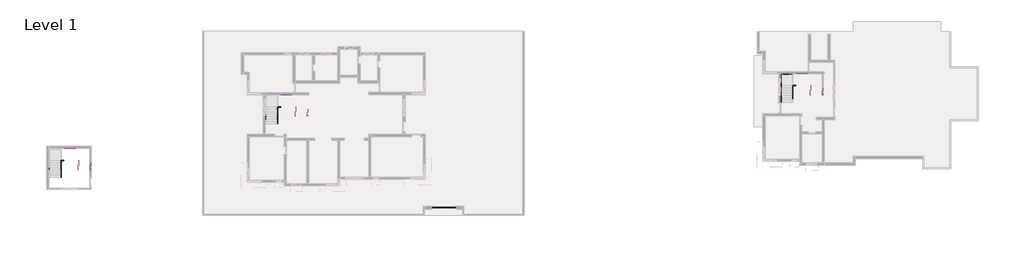
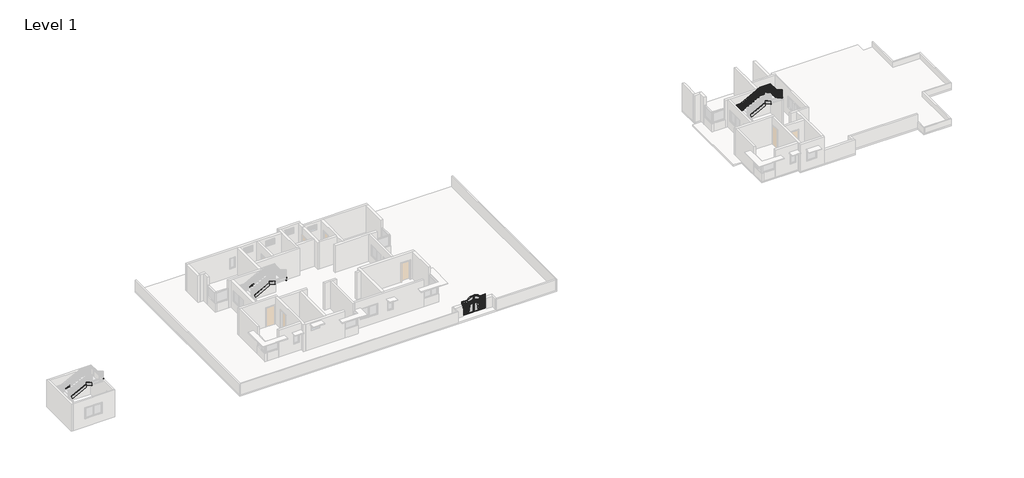
# One storey, part 9 of 9: 18 members, 1 proxy, 1 railing.
"""IFC4 building model written with IfcOpenShell, lengths in millimetres."""

from ifc_helpers import new_model, si_unit, frame, origin, place, context, project, spatial, polyline, outline, extrude, faceted_brep, transform, mapped, element, save
from components import generic_models_6bc30956

model = new_model("IFC4")

# Units and contexts
model_context = context("Model", 3, world=origin())
ifc_project = project(units=[si_unit("LENGTHUNIT", "METRE", prefix="MILLI")], contexts=[model_context])

# Site, building, storey
site = spatial("IfcSite", under=ifc_project)
building = spatial("IfcBuilding", under=site)
storey = spatial("IfcBuildingStorey", under=building, Name="Level 1", Elevation=0.0)

# Proxy
placement = place(None, origin())
generic_models_shape = generic_models_6bc30956(model_context)
element("IfcBuildingElementProxy", 1, Name="Generic Models", at=placement, inside=storey, context=model_context, shape_type="MappedRepresentation", body=[
    mapped(generic_models_shape, transform((-22180.3146233, 3588.8624892, 0.0), x_axis=(1.0, 0.0, 0.0), y_axis=(0.0, 1.0, 0.0), z_axis=(0.0, 0.0, 1.0))),
])

# Members
element("IfcMember", 2, ObjectType="Stringer - 2\" Width", at=placement, inside=storey, context=model_context, shape_type="SweptSolid", body=[
    extrude(outline(polyline([(14647.8480703, 0.0), (14647.8480703, 208.974685), (15536.2673716, 716.6428571), (16150.6114121, 716.6428571), (14896.4864121, 0.0), (14647.8480703, 0.0)])), frame((13242.1100959, 0.0, 0.0), z_axis=(1.0, 0.0, 0.0), x_axis=(0.0, 1.0, 0.0)), (0.0, 0.0, 1.0), 50.8),
])
element("IfcMember", 3, ObjectType="Stringer - 2\" Width", at=placement, inside=storey, context=model_context, shape_type="SweptSolid", body=[
    extrude(outline(polyline([(1570.6066619, 15541.7922297), (1834.574685, 16036.732273), (1834.574685, 15389.032273), (1570.6066619, 14894.0922297), (1570.6066619, 15541.7922297)])), frame((0.0, 17645.0480703, 0.0), z_axis=(0.0, 1.0, 0.0), x_axis=(0.0, 0.0, 1.0)), (0.0, 0.0, 1.0), 50.8),
])
element("IfcMember", 4, ObjectType="Stringer - 2\" Width", at=placement, inside=storey, context=model_context, shape_type="SweptSolid", body=[
    extrude(outline(polyline([(15537.7647285, 2687.6828571), (15409.8480703, 2760.7780904), (15409.8480703, 3111.8318278), (16152.108769, 2687.6828571), (15537.7647285, 2687.6828571)])), frame((17636.3100959, 0.0, 0.0), z_axis=(1.0, 0.0, 0.0), x_axis=(0.0, 1.0, 0.0)), (0.0, 0.0, 1.0), 50.8),
])
element("IfcMember", 5, ObjectType="Stringer - 2\" Width", at=placement, inside=storey, context=model_context, shape_type="SweptSolid", body=[
    extrude(outline(polyline([(14647.8480703, 0.0), (14647.8480703, 208.974685), (16375.0480703, 1195.9461135), (16375.0480703, 844.8923761), (14896.4864121, 0.0), (14647.8480703, 0.0)])), frame((14512.1100959, 0.0, 0.0), z_axis=(1.0, 0.0, 0.0), x_axis=(0.0, 1.0, 0.0)), (0.0, 0.0, 1.0), 50.8),
])
element("IfcMember", 6, ObjectType="Stringer - 2\" Width", at=placement, inside=storey, context=model_context, shape_type="SweptSolid", body=[
    extrude(outline(polyline([(1366.8828571, 14512.1100959), (1021.4428571, 14512.1100959), (2010.3495238, 16366.3100959), (2355.7895238, 16366.3100959), (1366.8828571, 14512.1100959)])), frame((0.0, 16375.0480703, 0.0), z_axis=(0.0, 1.0, 0.0), x_axis=(0.0, 0.0, 1.0)), (0.0, 0.0, 1.0), 50.8),
])
element("IfcMember", 7, ObjectType="Stringer - 2\" Width", at=placement, inside=storey, context=model_context, shape_type="SweptSolid", body=[
    extrude(outline(polyline([(16425.8480703, 2531.2603992), (16425.8480703, 2180.2066619), (15409.8480703, 2760.7780904), (15409.8480703, 3111.8318278), (16425.8480703, 2531.2603992)])), frame((16366.3100959, 0.0, 0.0), z_axis=(1.0, 0.0, 0.0), x_axis=(0.0, 1.0, 0.0)), (0.0, 0.0, 1.0), 50.8),
])
element("IfcMember", 8, ObjectType="Stringer - 2\" Width", at=placement, inside=storey, context=model_context, shape_type="SweptSolid", body=[
    extrude(outline(polyline([(12415.3624892, 0.0), (12415.3624892, 208.974685), (13303.7817906, 716.6428571), (13918.125831, 716.6428571), (12664.000831, 0.0), (12415.3624892, 0.0)])), frame((-41001.7146233, 0.0, 0.0), z_axis=(1.0, 0.0, 0.0), x_axis=(0.0, 1.0, 0.0)), (0.0, 0.0, 1.0), 50.8),
])
element("IfcMember", 9, ObjectType="Stringer - 2\" Width", at=placement, inside=storey, context=model_context, shape_type="SweptSolid", body=[
    extrude(outline(polyline([(1570.6066619, -38702.0324895), (1834.574685, -38207.0924462), (1834.574685, -38854.7924462), (1570.6066619, -39349.7324895), (1570.6066619, -38702.0324895)])), frame((0.0, 15412.5624892, 0.0), z_axis=(0.0, 1.0, 0.0), x_axis=(0.0, 0.0, 1.0)), (0.0, 0.0, 1.0), 50.8),
])
element("IfcMember", 10, ObjectType="Stringer - 2\" Width", at=placement, inside=storey, context=model_context, shape_type="SweptSolid", body=[
    extrude(outline(polyline([(13305.2791475, 2687.6828571), (13177.3624892, 2760.7780904), (13177.3624892, 3111.8318278), (13919.6231879, 2687.6828571), (13305.2791475, 2687.6828571)])), frame((-36607.5146233, 0.0, 0.0), z_axis=(1.0, 0.0, 0.0), x_axis=(0.0, 1.0, 0.0)), (0.0, 0.0, 1.0), 50.8),
])
element("IfcMember", 11, ObjectType="Stringer - 2\" Width", at=placement, inside=storey, context=model_context, shape_type="SweptSolid", body=[
    extrude(outline(polyline([(12415.3624892, 0.0), (12415.3624892, 208.974685), (14142.5624892, 1195.9461135), (14142.5624892, 844.8923761), (12664.000831, 0.0), (12415.3624892, 0.0)])), frame((-39731.7146233, 0.0, 0.0), z_axis=(1.0, 0.0, 0.0), x_axis=(0.0, 1.0, 0.0)), (0.0, 0.0, 1.0), 50.8),
])
element("IfcMember", 12, ObjectType="Stringer - 2\" Width", at=placement, inside=storey, context=model_context, shape_type="SweptSolid", body=[
    extrude(outline(polyline([(1366.8828571, -39731.7146233), (1021.4428571, -39731.7146233), (2010.3495238, -37877.5146233), (2355.7895238, -37877.5146233), (1366.8828571, -39731.7146233)])), frame((0.0, 14142.5624892, 0.0), z_axis=(0.0, 1.0, 0.0), x_axis=(0.0, 0.0, 1.0)), (0.0, 0.0, 1.0), 50.8),
])
element("IfcMember", 13, ObjectType="Stringer - 2\" Width", at=placement, inside=storey, context=model_context, shape_type="SweptSolid", body=[
    extrude(outline(polyline([(14193.3624892, 2531.2603992), (14193.3624892, 2180.2066619), (13177.3624892, 2760.7780904), (13177.3624892, 3111.8318278), (14193.3624892, 2531.2603992)])), frame((-37877.5146233, 0.0, 0.0), z_axis=(1.0, 0.0, 0.0), x_axis=(0.0, 1.0, 0.0)), (0.0, 0.0, 1.0), 50.8),
])
element("IfcMember", 14, ObjectType="Stringer - 2\" Width", at=placement, inside=storey, context=model_context, shape_type="SweptSolid", body=[
    extrude(outline(polyline([(6754.3199577, 0.0), (6754.3199577, 208.974685), (7642.739259, 716.6428571), (8257.0832994, 716.6428571), (7002.9582994, 0.0), (6754.3199577, 0.0)])), frame((-63814.6636189, 0.0, 0.0), z_axis=(1.0, 0.0, 0.0), x_axis=(0.0, 1.0, 0.0)), (0.0, 0.0, 1.0), 50.8),
])
element("IfcMember", 15, ObjectType="Stringer - 2\" Width", at=placement, inside=storey, context=model_context, shape_type="SweptSolid", body=[
    extrude(outline(polyline([(1570.6066619, -61514.981485), (1834.574685, -61020.0414417), (1834.574685, -61667.7414417), (1570.6066619, -62162.681485), (1570.6066619, -61514.981485)])), frame((0.0, 9751.5199577, 0.0), z_axis=(0.0, 1.0, 0.0), x_axis=(0.0, 0.0, 1.0)), (0.0, 0.0, 1.0), 50.8),
])
element("IfcMember", 16, ObjectType="Stringer - 2\" Width", at=placement, inside=storey, context=model_context, shape_type="SweptSolid", body=[
    extrude(outline(polyline([(7644.2366159, 2687.6828571), (7516.3199577, 2760.7780904), (7516.3199577, 3111.8318278), (8258.5806563, 2687.6828571), (7644.2366159, 2687.6828571)])), frame((-59420.4636189, 0.0, 0.0), z_axis=(1.0, 0.0, 0.0), x_axis=(0.0, 1.0, 0.0)), (0.0, 0.0, 1.0), 50.8),
])
element("IfcMember", 17, ObjectType="Stringer - 2\" Width", at=placement, inside=storey, context=model_context, shape_type="SweptSolid", body=[
    extrude(outline(polyline([(6754.3199577, 0.0), (6754.3199577, 208.974685), (8481.5199577, 1195.9461135), (8481.5199577, 844.8923761), (7002.9582994, 0.0), (6754.3199577, 0.0)])), frame((-62544.6636189, 0.0, 0.0), z_axis=(1.0, 0.0, 0.0), x_axis=(0.0, 1.0, 0.0)), (0.0, 0.0, 1.0), 50.8),
])
element("IfcMember", 18, ObjectType="Stringer - 2\" Width", at=placement, inside=storey, context=model_context, shape_type="SweptSolid", body=[
    extrude(outline(polyline([(1366.8828571, -62544.6636189), (1021.4428571, -62544.6636189), (2010.3495238, -60690.4636189), (2355.7895238, -60690.4636189), (1366.8828571, -62544.6636189)])), frame((0.0, 8481.5199577, 0.0), z_axis=(0.0, 1.0, 0.0), x_axis=(0.0, 0.0, 1.0)), (0.0, 0.0, 1.0), 50.8),
])
element("IfcMember", 19, ObjectType="Stringer - 2\" Width", at=placement, inside=storey, context=model_context, shape_type="SweptSolid", body=[
    extrude(outline(polyline([(8532.3199577, 2531.2603992), (8532.3199577, 2180.2066619), (7516.3199577, 2760.7780904), (7516.3199577, 3111.8318278), (8532.3199577, 2531.2603992)])), frame((-60690.4636189, 0.0, 0.0), z_axis=(1.0, 0.0, 0.0), x_axis=(0.0, 1.0, 0.0)), (0.0, 0.0, 1.0), 50.8),
])

# Railing
element("IfcRailing", 20, ObjectType="Handrail - Rectangular", at=placement, inside=storey, context=model_context, shape_type="SolidModel", body=[
    faceted_brep([(13292.9100959, 14647.8480703, 1059.5428571), (13292.9100959, 14647.8480703, 1001.0339009), (13343.7100959, 14647.8480703, 1001.0339009), (13343.7100959, 14647.8480703, 1059.5428571), (13292.9100959, 16592.6414036, 2170.8533333), (13292.9100959, 16606.132077, 2120.0533333), (13343.7100959, 16606.132077, 2120.0533333), (13343.7100959, 16592.6414036, 2170.8533333), (13292.9100959, 17645.0480703, 2170.8533333), (13292.9100959, 17645.0480703, 2120.0533333), (13343.7100959, 17594.2480703, 2120.0533333), (13343.7100959, 17594.2480703, 2170.8533333), (14418.6743816, 17645.0480703, 2170.8533333), (14431.3743816, 17645.0480703, 2120.0533333), (14431.3743816, 17594.2480703, 2120.0533333), (14418.6743816, 17594.2480703, 2170.8533333), (16510.5458102, 17645.0480703, 3286.5180952), (16523.2458102, 17645.0480703, 3235.7180952), (16523.2458102, 17594.2480703, 3235.7180952), (16510.5458102, 17594.2480703, 3286.5180952), (17636.3100959, 17645.0480703, 3286.5180952), (17636.3100959, 17645.0480703, 3235.7180952), (17585.5100959, 17594.2480703, 3235.7180952), (17585.5100959, 17594.2480703, 3286.5180952), (17636.3100959, 16592.6414036, 3286.5180952), (17636.3100959, 16579.1507302, 3235.7180952), (17585.5100959, 16579.1507302, 3235.7180952), (17585.5100959, 16592.6414036, 3286.5180952), (17636.3100959, 15409.8480703, 3962.4), (17585.5100959, 15409.8480703, 3962.4), (17585.5100959, 15409.8480703, 3903.8910438), (17636.3100959, 15409.8480703, 3903.8910438)], [[[0, 1, 2, 3]], [[1, 0, 4, 5]], [[2, 1, 5, 6]], [[3, 2, 6, 7]], [[0, 3, 7, 4]], [[5, 4, 8, 9]], [[6, 5, 9, 10]], [[7, 6, 10, 11]], [[4, 7, 11, 8]], [[9, 8, 12, 13]], [[10, 9, 13, 14]], [[11, 10, 14, 15]], [[8, 11, 15, 12]], [[13, 12, 16, 17]], [[14, 13, 17, 18]], [[15, 14, 18, 19]], [[12, 15, 19, 16]], [[17, 16, 20, 21]], [[18, 17, 21, 22]], [[19, 18, 22, 23]], [[16, 19, 23, 20]], [[21, 20, 24, 25]], [[22, 21, 25, 26]], [[23, 22, 26, 27]], [[20, 23, 27, 24]], [[28, 29, 30, 31]], [[25, 24, 28, 31]], [[26, 25, 31, 30]], [[27, 26, 30, 29]], [[24, 27, 29, 28]]]),
    extrude(outline(polyline([(15495.5730703, 3854.9053295), (15495.5730703, 2902.8571429), (15476.5230703, 2902.8571429), (15476.5230703, 3865.7910438), (15495.5730703, 3854.9053295)])), frame((17601.3850959, 0.0, 0.0), z_axis=(1.0, 0.0, 0.0), x_axis=(0.0, 1.0, 0.0)), (0.0, 0.0, 1.0), 19.05),
    extrude(outline(polyline([(15597.1730703, 3796.8481866), (15597.1730703, 2902.8571429), (15578.1230703, 2902.8571429), (15578.1230703, 3807.7339009), (15597.1730703, 3796.8481866)])), frame((17601.3850959, 0.0, 0.0), z_axis=(1.0, 0.0, 0.0), x_axis=(0.0, 1.0, 0.0)), (0.0, 0.0, 1.0), 19.05),
    extrude(outline(polyline([(15698.7730703, 3738.7910438), (15698.7730703, 2757.7142857), (15679.7230703, 2757.7142857), (15679.7230703, 3749.6767581), (15698.7730703, 3738.7910438)])), frame((17601.3850959, 0.0, 0.0), z_axis=(1.0, 0.0, 0.0), x_axis=(0.0, 1.0, 0.0)), (0.0, 0.0, 1.0), 19.05),
    extrude(outline(polyline([(15800.3730703, 3680.7339009), (15800.3730703, 2757.7142857), (15781.3230703, 2757.7142857), (15781.3230703, 3691.6196152), (15800.3730703, 3680.7339009)])), frame((17601.3850959, 0.0, 0.0), z_axis=(1.0, 0.0, 0.0), x_axis=(0.0, 1.0, 0.0)), (0.0, 0.0, 1.0), 19.05),
    extrude(outline(polyline([(15901.9730703, 3622.6767581), (15901.9730703, 2757.7142857), (15882.9230703, 2757.7142857), (15882.9230703, 3633.5624723), (15901.9730703, 3622.6767581)])), frame((17601.3850959, 0.0, 0.0), z_axis=(1.0, 0.0, 0.0), x_axis=(0.0, 1.0, 0.0)), (0.0, 0.0, 1.0), 19.05),
    extrude(outline(polyline([(16003.5730703, 3564.6196152), (16003.5730703, 2612.5714286), (15984.5230703, 2612.5714286), (15984.5230703, 3575.5053295), (16003.5730703, 3564.6196152)])), frame((17601.3850959, 0.0, 0.0), z_axis=(1.0, 0.0, 0.0), x_axis=(0.0, 1.0, 0.0)), (0.0, 0.0, 1.0), 19.05),
    extrude(outline(polyline([(16105.1730703, 3506.5624723), (16105.1730703, 2612.5714286), (16086.1230703, 2612.5714286), (16086.1230703, 3517.4481866), (16105.1730703, 3506.5624723)])), frame((17601.3850959, 0.0, 0.0), z_axis=(1.0, 0.0, 0.0), x_axis=(0.0, 1.0, 0.0)), (0.0, 0.0, 1.0), 19.05),
    extrude(outline(polyline([(16206.7730703, 3448.5053295), (16206.7730703, 2467.4285714), (16187.7230703, 2467.4285714), (16187.7230703, 3459.3910438), (16206.7730703, 3448.5053295)])), frame((17601.3850959, 0.0, 0.0), z_axis=(1.0, 0.0, 0.0), x_axis=(0.0, 1.0, 0.0)), (0.0, 0.0, 1.0), 19.05),
    extrude(outline(polyline([(16308.3730703, 3390.4481866), (16308.3730703, 2467.4285714), (16289.3230703, 2467.4285714), (16289.3230703, 3401.3339009), (16308.3730703, 3390.4481866)])), frame((17601.3850959, 0.0, 0.0), z_axis=(1.0, 0.0, 0.0), x_axis=(0.0, 1.0, 0.0)), (0.0, 0.0, 1.0), 19.05),
    extrude(outline(polyline([(16409.9730703, 3332.3910438), (16409.9730703, 2467.4285714), (16390.9230703, 2467.4285714), (16390.9230703, 3343.2767581), (16409.9730703, 3332.3910438)])), frame((17601.3850959, 0.0, 0.0), z_axis=(1.0, 0.0, 0.0), x_axis=(0.0, 1.0, 0.0)), (0.0, 0.0, 1.0), 19.05),
    extrude(outline(polyline([(16511.5730703, 3274.3339009), (16511.5730703, 2322.2857143), (16492.5230703, 2322.2857143), (16492.5230703, 3285.2196152), (16511.5730703, 3274.3339009)])), frame((17601.3850959, 0.0, 0.0), z_axis=(1.0, 0.0, 0.0), x_axis=(0.0, 1.0, 0.0)), (0.0, 0.0, 1.0), 19.05),
    extrude(outline(polyline([(17620.4350959, 16613.1730703), (17620.4350959, 16594.1230703), (17601.3850959, 16594.1230703), (17601.3850959, 16613.1730703), (17620.4350959, 16613.1730703)])), frame((0.0, 0.0, 2322.2857143), z_axis=(0.0, 0.0, 1.0), x_axis=(1.0, 0.0, 0.0)), (0.0, 0.0, 1.0), 913.432381),
    extrude(outline(polyline([(17620.4350959, 16714.7730703), (17620.4350959, 16695.7230703), (17601.3850959, 16695.7230703), (17601.3850959, 16714.7730703), (17620.4350959, 16714.7730703)])), frame((0.0, 0.0, 2322.2857143), z_axis=(0.0, 0.0, 1.0), x_axis=(1.0, 0.0, 0.0)), (0.0, 0.0, 1.0), 913.432381),
    extrude(outline(polyline([(17620.4350959, 16816.3730703), (17620.4350959, 16797.3230703), (17601.3850959, 16797.3230703), (17601.3850959, 16816.3730703), (17620.4350959, 16816.3730703)])), frame((0.0, 0.0, 2322.2857143), z_axis=(0.0, 0.0, 1.0), x_axis=(1.0, 0.0, 0.0)), (0.0, 0.0, 1.0), 913.432381),
    extrude(outline(polyline([(17620.4350959, 16917.9730703), (17620.4350959, 16898.9230703), (17601.3850959, 16898.9230703), (17601.3850959, 16917.9730703), (17620.4350959, 16917.9730703)])), frame((0.0, 0.0, 2322.2857143), z_axis=(0.0, 0.0, 1.0), x_axis=(1.0, 0.0, 0.0)), (0.0, 0.0, 1.0), 913.432381),
    extrude(outline(polyline([(17620.4350959, 17019.5730703), (17620.4350959, 17000.5230703), (17601.3850959, 17000.5230703), (17601.3850959, 17019.5730703), (17620.4350959, 17019.5730703)])), frame((0.0, 0.0, 2322.2857143), z_axis=(0.0, 0.0, 1.0), x_axis=(1.0, 0.0, 0.0)), (0.0, 0.0, 1.0), 913.432381),
    extrude(outline(polyline([(17620.4350959, 17121.1730703), (17620.4350959, 17102.1230703), (17601.3850959, 17102.1230703), (17601.3850959, 17121.1730703), (17620.4350959, 17121.1730703)])), frame((0.0, 0.0, 2322.2857143), z_axis=(0.0, 0.0, 1.0), x_axis=(1.0, 0.0, 0.0)), (0.0, 0.0, 1.0), 913.432381),
    extrude(outline(polyline([(17620.4350959, 17222.7730703), (17620.4350959, 17203.7230703), (17601.3850959, 17203.7230703), (17601.3850959, 17222.7730703), (17620.4350959, 17222.7730703)])), frame((0.0, 0.0, 2322.2857143), z_axis=(0.0, 0.0, 1.0), x_axis=(1.0, 0.0, 0.0)), (0.0, 0.0, 1.0), 913.432381),
    extrude(outline(polyline([(17620.4350959, 17324.3730703), (17620.4350959, 17305.3230703), (17601.3850959, 17305.3230703), (17601.3850959, 17324.3730703), (17620.4350959, 17324.3730703)])), frame((0.0, 0.0, 2322.2857143), z_axis=(0.0, 0.0, 1.0), x_axis=(1.0, 0.0, 0.0)), (0.0, 0.0, 1.0), 913.432381),
    extrude(outline(polyline([(17620.4350959, 17425.9730703), (17620.4350959, 17406.9230703), (17601.3850959, 17406.9230703), (17601.3850959, 17425.9730703), (17620.4350959, 17425.9730703)])), frame((0.0, 0.0, 2322.2857143), z_axis=(0.0, 0.0, 1.0), x_axis=(1.0, 0.0, 0.0)), (0.0, 0.0, 1.0), 913.432381),
    extrude(outline(polyline([(17620.4350959, 17527.5730703), (17620.4350959, 17508.5230703), (17601.3850959, 17508.5230703), (17601.3850959, 17527.5730703), (17620.4350959, 17527.5730703)])), frame((0.0, 0.0, 2322.2857143), z_axis=(0.0, 0.0, 1.0), x_axis=(1.0, 0.0, 0.0)), (0.0, 0.0, 1.0), 913.432381),
    extrude(outline(polyline([(17575.9850959, 17629.1730703), (17595.0350959, 17629.1730703), (17595.0350959, 17610.1230703), (17575.9850959, 17610.1230703), (17575.9850959, 17629.1730703)])), frame((0.0, 0.0, 2322.2857143), z_axis=(0.0, 0.0, 1.0), x_axis=(1.0, 0.0, 0.0)), (0.0, 0.0, 1.0), 913.432381),
    extrude(outline(polyline([(17474.3850959, 17629.1730703), (17493.4350959, 17629.1730703), (17493.4350959, 17610.1230703), (17474.3850959, 17610.1230703), (17474.3850959, 17629.1730703)])), frame((0.0, 0.0, 2322.2857143), z_axis=(0.0, 0.0, 1.0), x_axis=(1.0, 0.0, 0.0)), (0.0, 0.0, 1.0), 913.432381),
    extrude(outline(polyline([(17372.7850959, 17629.1730703), (17391.8350959, 17629.1730703), (17391.8350959, 17610.1230703), (17372.7850959, 17610.1230703), (17372.7850959, 17629.1730703)])), frame((0.0, 0.0, 2322.2857143), z_axis=(0.0, 0.0, 1.0), x_axis=(1.0, 0.0, 0.0)), (0.0, 0.0, 1.0), 913.432381),
    extrude(outline(polyline([(17271.1850959, 17629.1730703), (17290.2350959, 17629.1730703), (17290.2350959, 17610.1230703), (17271.1850959, 17610.1230703), (17271.1850959, 17629.1730703)])), frame((0.0, 0.0, 2322.2857143), z_axis=(0.0, 0.0, 1.0), x_axis=(1.0, 0.0, 0.0)), (0.0, 0.0, 1.0), 913.432381),
    extrude(outline(polyline([(17169.5850959, 17629.1730703), (17188.6350959, 17629.1730703), (17188.6350959, 17610.1230703), (17169.5850959, 17610.1230703), (17169.5850959, 17629.1730703)])), frame((0.0, 0.0, 2322.2857143), z_axis=(0.0, 0.0, 1.0), x_axis=(1.0, 0.0, 0.0)), (0.0, 0.0, 1.0), 913.432381),
    extrude(outline(polyline([(17067.9850959, 17629.1730703), (17087.0350959, 17629.1730703), (17087.0350959, 17610.1230703), (17067.9850959, 17610.1230703), (17067.9850959, 17629.1730703)])), frame((0.0, 0.0, 2322.2857143), z_axis=(0.0, 0.0, 1.0), x_axis=(1.0, 0.0, 0.0)), (0.0, 0.0, 1.0), 913.432381),
    extrude(outline(polyline([(16966.3850959, 17629.1730703), (16985.4350959, 17629.1730703), (16985.4350959, 17610.1230703), (16966.3850959, 17610.1230703), (16966.3850959, 17629.1730703)])), frame((0.0, 0.0, 2322.2857143), z_axis=(0.0, 0.0, 1.0), x_axis=(1.0, 0.0, 0.0)), (0.0, 0.0, 1.0), 913.432381),
    extrude(outline(polyline([(16864.7850959, 17629.1730703), (16883.8350959, 17629.1730703), (16883.8350959, 17610.1230703), (16864.7850959, 17610.1230703), (16864.7850959, 17629.1730703)])), frame((0.0, 0.0, 2322.2857143), z_axis=(0.0, 0.0, 1.0), x_axis=(1.0, 0.0, 0.0)), (0.0, 0.0, 1.0), 913.432381),
    extrude(outline(polyline([(16763.1850959, 17629.1730703), (16782.2350959, 17629.1730703), (16782.2350959, 17610.1230703), (16763.1850959, 17610.1230703), (16763.1850959, 17629.1730703)])), frame((0.0, 0.0, 2322.2857143), z_axis=(0.0, 0.0, 1.0), x_axis=(1.0, 0.0, 0.0)), (0.0, 0.0, 1.0), 913.432381),
    extrude(outline(polyline([(16661.5850959, 17629.1730703), (16680.6350959, 17629.1730703), (16680.6350959, 17610.1230703), (16661.5850959, 17610.1230703), (16661.5850959, 17629.1730703)])), frame((0.0, 0.0, 2322.2857143), z_axis=(0.0, 0.0, 1.0), x_axis=(1.0, 0.0, 0.0)), (0.0, 0.0, 1.0), 913.432381),
    extrude(outline(polyline([(16559.9850959, 17629.1730703), (16579.0350959, 17629.1730703), (16579.0350959, 17610.1230703), (16559.9850959, 17610.1230703), (16559.9850959, 17629.1730703)])), frame((0.0, 0.0, 2322.2857143), z_axis=(0.0, 0.0, 1.0), x_axis=(1.0, 0.0, 0.0)), (0.0, 0.0, 1.0), 913.432381),
    extrude(outline(polyline([(3201.1257143, 16458.3850959), (2322.2857143, 16458.3850959), (2322.2857143, 16477.4350959), (3211.2857143, 16477.4350959), (3201.1257143, 16458.3850959)])), frame((0.0, 17610.1230703, 0.0), z_axis=(0.0, 1.0, 0.0), x_axis=(0.0, 0.0, 1.0)), (0.0, 0.0, 1.0), 19.05),
    extrude(outline(polyline([(3146.9390476, 16356.7850959), (2177.1428571, 16356.7850959), (2177.1428571, 16375.8350959), (3157.0990476, 16375.8350959), (3146.9390476, 16356.7850959)])), frame((0.0, 17610.1230703, 0.0), z_axis=(0.0, 1.0, 0.0), x_axis=(0.0, 0.0, 1.0)), (0.0, 0.0, 1.0), 19.05),
    extrude(outline(polyline([(3092.752381, 16255.1850959), (2177.1428571, 16255.1850959), (2177.1428571, 16274.2350959), (3102.912381, 16274.2350959), (3092.752381, 16255.1850959)])), frame((0.0, 17610.1230703, 0.0), z_axis=(0.0, 1.0, 0.0), x_axis=(0.0, 0.0, 1.0)), (0.0, 0.0, 1.0), 19.05),
    extrude(outline(polyline([(3038.5657143, 16153.5850959), (2177.1428571, 16153.5850959), (2177.1428571, 16172.6350959), (3048.7257143, 16172.6350959), (3038.5657143, 16153.5850959)])), frame((0.0, 17610.1230703, 0.0), z_axis=(0.0, 1.0, 0.0), x_axis=(0.0, 0.0, 1.0)), (0.0, 0.0, 1.0), 19.05),
    extrude(outline(polyline([(2984.3790476, 16051.9850959), (2032.0, 16051.9850959), (2032.0, 16071.0350959), (2994.5390476, 16071.0350959), (2984.3790476, 16051.9850959)])), frame((0.0, 17610.1230703, 0.0), z_axis=(0.0, 1.0, 0.0), x_axis=(0.0, 0.0, 1.0)), (0.0, 0.0, 1.0), 19.05),
    extrude(outline(polyline([(2930.192381, 15950.3850959), (2032.0, 15950.3850959), (2032.0, 15969.4350959), (2940.352381, 15969.4350959), (2930.192381, 15950.3850959)])), frame((0.0, 17610.1230703, 0.0), z_axis=(0.0, 1.0, 0.0), x_axis=(0.0, 0.0, 1.0)), (0.0, 0.0, 1.0), 19.05),
    extrude(outline(polyline([(2876.0057143, 15848.7850959), (1886.8571429, 15848.7850959), (1886.8571429, 15867.8350959), (2886.1657143, 15867.8350959), (2876.0057143, 15848.7850959)])), frame((0.0, 17610.1230703, 0.0), z_axis=(0.0, 1.0, 0.0), x_axis=(0.0, 0.0, 1.0)), (0.0, 0.0, 1.0), 19.05),
    extrude(outline(polyline([(2821.8190476, 15747.1850959), (1886.8571429, 15747.1850959), (1886.8571429, 15766.2350959), (2831.9790476, 15766.2350959), (2821.8190476, 15747.1850959)])), frame((0.0, 17610.1230703, 0.0), z_axis=(0.0, 1.0, 0.0), x_axis=(0.0, 0.0, 1.0)), (0.0, 0.0, 1.0), 19.05),
    extrude(outline(polyline([(2767.632381, 15645.5850959), (1886.8571429, 15645.5850959), (1886.8571429, 15664.6350959), (2777.792381, 15664.6350959), (2767.632381, 15645.5850959)])), frame((0.0, 17610.1230703, 0.0), z_axis=(0.0, 1.0, 0.0), x_axis=(0.0, 0.0, 1.0)), (0.0, 0.0, 1.0), 19.05),
    extrude(outline(polyline([(2713.4457143, 15543.9850959), (1741.7142857, 15543.9850959), (1741.7142857, 15563.0350959), (2723.6057143, 15563.0350959), (2713.4457143, 15543.9850959)])), frame((0.0, 17610.1230703, 0.0), z_axis=(0.0, 1.0, 0.0), x_axis=(0.0, 0.0, 1.0)), (0.0, 0.0, 1.0), 19.05),
    extrude(outline(polyline([(2659.2590476, 15442.3850959), (1741.7142857, 15442.3850959), (1741.7142857, 15461.4350959), (2669.4190476, 15461.4350959), (2659.2590476, 15442.3850959)])), frame((0.0, 17610.1230703, 0.0), z_axis=(0.0, 1.0, 0.0), x_axis=(0.0, 0.0, 1.0)), (0.0, 0.0, 1.0), 19.05),
    extrude(outline(polyline([(2605.072381, 15340.7850959), (1741.7142857, 15340.7850959), (1741.7142857, 15359.8350959), (2615.232381, 15359.8350959), (2605.072381, 15340.7850959)])), frame((0.0, 17610.1230703, 0.0), z_axis=(0.0, 1.0, 0.0), x_axis=(0.0, 0.0, 1.0)), (0.0, 0.0, 1.0), 19.05),
    extrude(outline(polyline([(2550.8857143, 15239.1850959), (1596.5714286, 15239.1850959), (1596.5714286, 15258.2350959), (2561.0457143, 15258.2350959), (2550.8857143, 15239.1850959)])), frame((0.0, 17610.1230703, 0.0), z_axis=(0.0, 1.0, 0.0), x_axis=(0.0, 0.0, 1.0)), (0.0, 0.0, 1.0), 19.05),
    extrude(outline(polyline([(2496.6990476, 15137.5850959), (1596.5714286, 15137.5850959), (1596.5714286, 15156.6350959), (2506.8590476, 15156.6350959), (2496.6990476, 15137.5850959)])), frame((0.0, 17610.1230703, 0.0), z_axis=(0.0, 1.0, 0.0), x_axis=(0.0, 0.0, 1.0)), (0.0, 0.0, 1.0), 19.05),
    extrude(outline(polyline([(2442.512381, 15035.9850959), (1596.5714286, 15035.9850959), (1596.5714286, 15055.0350959), (2452.672381, 15055.0350959), (2442.512381, 15035.9850959)])), frame((0.0, 17610.1230703, 0.0), z_axis=(0.0, 1.0, 0.0), x_axis=(0.0, 0.0, 1.0)), (0.0, 0.0, 1.0), 19.05),
    extrude(outline(polyline([(2388.3257143, 14934.3850959), (1451.4285714, 14934.3850959), (1451.4285714, 14953.4350959), (2398.4857143, 14953.4350959), (2388.3257143, 14934.3850959)])), frame((0.0, 17610.1230703, 0.0), z_axis=(0.0, 1.0, 0.0), x_axis=(0.0, 0.0, 1.0)), (0.0, 0.0, 1.0), 19.05),
    extrude(outline(polyline([(2334.1390476, 14832.7850959), (1451.4285714, 14832.7850959), (1451.4285714, 14851.8350959), (2344.2990476, 14851.8350959), (2334.1390476, 14832.7850959)])), frame((0.0, 17610.1230703, 0.0), z_axis=(0.0, 1.0, 0.0), x_axis=(0.0, 0.0, 1.0)), (0.0, 0.0, 1.0), 19.05),
    extrude(outline(polyline([(2279.952381, 14731.1850959), (1306.2857143, 14731.1850959), (1306.2857143, 14750.2350959), (2290.112381, 14750.2350959), (2279.952381, 14731.1850959)])), frame((0.0, 17610.1230703, 0.0), z_axis=(0.0, 1.0, 0.0), x_axis=(0.0, 0.0, 1.0)), (0.0, 0.0, 1.0), 19.05),
    extrude(outline(polyline([(2225.7657143, 14629.5850959), (1306.2857143, 14629.5850959), (1306.2857143, 14648.6350959), (2235.9257143, 14648.6350959), (2225.7657143, 14629.5850959)])), frame((0.0, 17610.1230703, 0.0), z_axis=(0.0, 1.0, 0.0), x_axis=(0.0, 0.0, 1.0)), (0.0, 0.0, 1.0), 19.05),
    extrude(outline(polyline([(2171.5790476, 14527.9850959), (1306.2857143, 14527.9850959), (1306.2857143, 14547.0350959), (2181.7390476, 14547.0350959), (2171.5790476, 14527.9850959)])), frame((0.0, 17610.1230703, 0.0), z_axis=(0.0, 1.0, 0.0), x_axis=(0.0, 0.0, 1.0)), (0.0, 0.0, 1.0), 19.05),
    extrude(outline(polyline([(2117.392381, 14426.3850959), (1161.1428571, 14426.3850959), (1161.1428571, 14445.4350959), (2127.552381, 14445.4350959), (2117.392381, 14426.3850959)])), frame((0.0, 17610.1230703, 0.0), z_axis=(0.0, 1.0, 0.0), x_axis=(0.0, 0.0, 1.0)), (0.0, 0.0, 1.0), 19.05),
    extrude(outline(polyline([(14324.7850959, 17629.1730703), (14343.8350959, 17629.1730703), (14343.8350959, 17610.1230703), (14324.7850959, 17610.1230703), (14324.7850959, 17629.1730703)])), frame((0.0, 0.0, 1161.1428571), z_axis=(0.0, 0.0, 1.0), x_axis=(1.0, 0.0, 0.0)), (0.0, 0.0, 1.0), 958.9104762),
    extrude(outline(polyline([(14223.1850959, 17629.1730703), (14242.2350959, 17629.1730703), (14242.2350959, 17610.1230703), (14223.1850959, 17610.1230703), (14223.1850959, 17629.1730703)])), frame((0.0, 0.0, 1161.1428571), z_axis=(0.0, 0.0, 1.0), x_axis=(1.0, 0.0, 0.0)), (0.0, 0.0, 1.0), 958.9104762),
    extrude(outline(polyline([(14121.5850959, 17629.1730703), (14140.6350959, 17629.1730703), (14140.6350959, 17610.1230703), (14121.5850959, 17610.1230703), (14121.5850959, 17629.1730703)])), frame((0.0, 0.0, 1161.1428571), z_axis=(0.0, 0.0, 1.0), x_axis=(1.0, 0.0, 0.0)), (0.0, 0.0, 1.0), 958.9104762),
    extrude(outline(polyline([(14019.9850959, 17629.1730703), (14039.0350959, 17629.1730703), (14039.0350959, 17610.1230703), (14019.9850959, 17610.1230703), (14019.9850959, 17629.1730703)])), frame((0.0, 0.0, 1161.1428571), z_axis=(0.0, 0.0, 1.0), x_axis=(1.0, 0.0, 0.0)), (0.0, 0.0, 1.0), 958.9104762),
    extrude(outline(polyline([(13918.3850959, 17629.1730703), (13937.4350959, 17629.1730703), (13937.4350959, 17610.1230703), (13918.3850959, 17610.1230703), (13918.3850959, 17629.1730703)])), frame((0.0, 0.0, 1161.1428571), z_axis=(0.0, 0.0, 1.0), x_axis=(1.0, 0.0, 0.0)), (0.0, 0.0, 1.0), 958.9104762),
    extrude(outline(polyline([(13816.7850959, 17629.1730703), (13835.8350959, 17629.1730703), (13835.8350959, 17610.1230703), (13816.7850959, 17610.1230703), (13816.7850959, 17629.1730703)])), frame((0.0, 0.0, 1161.1428571), z_axis=(0.0, 0.0, 1.0), x_axis=(1.0, 0.0, 0.0)), (0.0, 0.0, 1.0), 958.9104762),
    extrude(outline(polyline([(13715.1850959, 17629.1730703), (13734.2350959, 17629.1730703), (13734.2350959, 17610.1230703), (13715.1850959, 17610.1230703), (13715.1850959, 17629.1730703)])), frame((0.0, 0.0, 1161.1428571), z_axis=(0.0, 0.0, 1.0), x_axis=(1.0, 0.0, 0.0)), (0.0, 0.0, 1.0), 958.9104762),
    extrude(outline(polyline([(13613.5850959, 17629.1730703), (13632.6350959, 17629.1730703), (13632.6350959, 17610.1230703), (13613.5850959, 17610.1230703), (13613.5850959, 17629.1730703)])), frame((0.0, 0.0, 1161.1428571), z_axis=(0.0, 0.0, 1.0), x_axis=(1.0, 0.0, 0.0)), (0.0, 0.0, 1.0), 958.9104762),
    extrude(outline(polyline([(13511.9850959, 17629.1730703), (13531.0350959, 17629.1730703), (13531.0350959, 17610.1230703), (13511.9850959, 17610.1230703), (13511.9850959, 17629.1730703)])), frame((0.0, 0.0, 1161.1428571), z_axis=(0.0, 0.0, 1.0), x_axis=(1.0, 0.0, 0.0)), (0.0, 0.0, 1.0), 958.9104762),
    extrude(outline(polyline([(13410.3850959, 17629.1730703), (13429.4350959, 17629.1730703), (13429.4350959, 17610.1230703), (13410.3850959, 17610.1230703), (13410.3850959, 17629.1730703)])), frame((0.0, 0.0, 1161.1428571), z_axis=(0.0, 0.0, 1.0), x_axis=(1.0, 0.0, 0.0)), (0.0, 0.0, 1.0), 958.9104762),
    extrude(outline(polyline([(13308.7850959, 17584.7230703), (13308.7850959, 17603.7730703), (13327.8350959, 17603.7730703), (13327.8350959, 17584.7230703), (13308.7850959, 17584.7230703)])), frame((0.0, 0.0, 1161.1428571), z_axis=(0.0, 0.0, 1.0), x_axis=(1.0, 0.0, 0.0)), (0.0, 0.0, 1.0), 958.9104762),
    extrude(outline(polyline([(13308.7850959, 17483.1230703), (13308.7850959, 17502.1730703), (13327.8350959, 17502.1730703), (13327.8350959, 17483.1230703), (13308.7850959, 17483.1230703)])), frame((0.0, 0.0, 1161.1428571), z_axis=(0.0, 0.0, 1.0), x_axis=(1.0, 0.0, 0.0)), (0.0, 0.0, 1.0), 958.9104762),
    extrude(outline(polyline([(13308.7850959, 17381.5230703), (13308.7850959, 17400.5730703), (13327.8350959, 17400.5730703), (13327.8350959, 17381.5230703), (13308.7850959, 17381.5230703)])), frame((0.0, 0.0, 1161.1428571), z_axis=(0.0, 0.0, 1.0), x_axis=(1.0, 0.0, 0.0)), (0.0, 0.0, 1.0), 958.9104762),
    extrude(outline(polyline([(13308.7850959, 17279.9230703), (13308.7850959, 17298.9730703), (13327.8350959, 17298.9730703), (13327.8350959, 17279.9230703), (13308.7850959, 17279.9230703)])), frame((0.0, 0.0, 1161.1428571), z_axis=(0.0, 0.0, 1.0), x_axis=(1.0, 0.0, 0.0)), (0.0, 0.0, 1.0), 958.9104762),
    extrude(outline(polyline([(13308.7850959, 17178.3230703), (13308.7850959, 17197.3730703), (13327.8350959, 17197.3730703), (13327.8350959, 17178.3230703), (13308.7850959, 17178.3230703)])), frame((0.0, 0.0, 1161.1428571), z_axis=(0.0, 0.0, 1.0), x_axis=(1.0, 0.0, 0.0)), (0.0, 0.0, 1.0), 958.9104762),
    extrude(outline(polyline([(13308.7850959, 17076.7230703), (13308.7850959, 17095.7730703), (13327.8350959, 17095.7730703), (13327.8350959, 17076.7230703), (13308.7850959, 17076.7230703)])), frame((0.0, 0.0, 1161.1428571), z_axis=(0.0, 0.0, 1.0), x_axis=(1.0, 0.0, 0.0)), (0.0, 0.0, 1.0), 958.9104762),
    extrude(outline(polyline([(13308.7850959, 16975.1230703), (13308.7850959, 16994.1730703), (13327.8350959, 16994.1730703), (13327.8350959, 16975.1230703), (13308.7850959, 16975.1230703)])), frame((0.0, 0.0, 1161.1428571), z_axis=(0.0, 0.0, 1.0), x_axis=(1.0, 0.0, 0.0)), (0.0, 0.0, 1.0), 958.9104762),
    extrude(outline(polyline([(13308.7850959, 16873.5230703), (13308.7850959, 16892.5730703), (13327.8350959, 16892.5730703), (13327.8350959, 16873.5230703), (13308.7850959, 16873.5230703)])), frame((0.0, 0.0, 1161.1428571), z_axis=(0.0, 0.0, 1.0), x_axis=(1.0, 0.0, 0.0)), (0.0, 0.0, 1.0), 958.9104762),
    extrude(outline(polyline([(13308.7850959, 16771.9230703), (13308.7850959, 16790.9730703), (13327.8350959, 16790.9730703), (13327.8350959, 16771.9230703), (13308.7850959, 16771.9230703)])), frame((0.0, 0.0, 1161.1428571), z_axis=(0.0, 0.0, 1.0), x_axis=(1.0, 0.0, 0.0)), (0.0, 0.0, 1.0), 958.9104762),
    extrude(outline(polyline([(13308.7850959, 16670.3230703), (13308.7850959, 16689.3730703), (13327.8350959, 16689.3730703), (13327.8350959, 16670.3230703), (13308.7850959, 16670.3230703)])), frame((0.0, 0.0, 1161.1428571), z_axis=(0.0, 0.0, 1.0), x_axis=(1.0, 0.0, 0.0)), (0.0, 0.0, 1.0), 958.9104762),
    extrude(outline(polyline([(16587.7730703, 2109.5624723), (16587.7730703, 1161.1428571), (16568.7230703, 1161.1428571), (16568.7230703, 2098.6767581), (16587.7730703, 2109.5624723)])), frame((13308.7850959, 0.0, 0.0), z_axis=(1.0, 0.0, 0.0), x_axis=(0.0, 1.0, 0.0)), (0.0, 0.0, 1.0), 19.05),
    extrude(outline(polyline([(16486.1730703, 2051.5053295), (16486.1730703, 1161.1428571), (16467.1230703, 1161.1428571), (16467.1230703, 2040.6196152), (16486.1730703, 2051.5053295)])), frame((13308.7850959, 0.0, 0.0), z_axis=(1.0, 0.0, 0.0), x_axis=(0.0, 1.0, 0.0)), (0.0, 0.0, 1.0), 19.05),
    extrude(outline(polyline([(16384.5730703, 1993.4481866), (16384.5730703, 1016.0), (16365.5230703, 1016.0), (16365.5230703, 1982.5624723), (16384.5730703, 1993.4481866)])), frame((13308.7850959, 0.0, 0.0), z_axis=(1.0, 0.0, 0.0), x_axis=(0.0, 1.0, 0.0)), (0.0, 0.0, 1.0), 19.05),
    extrude(outline(polyline([(16282.9730703, 1935.3910438), (16282.9730703, 1016.0), (16263.9230703, 1016.0), (16263.9230703, 1924.5053295), (16282.9730703, 1935.3910438)])), frame((13308.7850959, 0.0, 0.0), z_axis=(1.0, 0.0, 0.0), x_axis=(0.0, 1.0, 0.0)), (0.0, 0.0, 1.0), 19.05),
    extrude(outline(polyline([(16181.3730703, 1877.3339009), (16181.3730703, 1016.0), (16162.3230703, 1016.0), (16162.3230703, 1866.4481866), (16181.3730703, 1877.3339009)])), frame((13308.7850959, 0.0, 0.0), z_axis=(1.0, 0.0, 0.0), x_axis=(0.0, 1.0, 0.0)), (0.0, 0.0, 1.0), 19.05),
    extrude(outline(polyline([(16079.7730703, 1819.2767581), (16079.7730703, 870.8571429), (16060.7230703, 870.8571429), (16060.7230703, 1808.3910438), (16079.7730703, 1819.2767581)])), frame((13308.7850959, 0.0, 0.0), z_axis=(1.0, 0.0, 0.0), x_axis=(0.0, 1.0, 0.0)), (0.0, 0.0, 1.0), 19.05),
    extrude(outline(polyline([(15978.1730703, 1761.2196152), (15978.1730703, 870.8571429), (15959.1230703, 870.8571429), (15959.1230703, 1750.3339009), (15978.1730703, 1761.2196152)])), frame((13308.7850959, 0.0, 0.0), z_axis=(1.0, 0.0, 0.0), x_axis=(0.0, 1.0, 0.0)), (0.0, 0.0, 1.0), 19.05),
    extrude(outline(polyline([(15876.5730703, 1703.1624723), (15876.5730703, 725.7142857), (15857.5230703, 725.7142857), (15857.5230703, 1692.2767581), (15876.5730703, 1703.1624723)])), frame((13308.7850959, 0.0, 0.0), z_axis=(1.0, 0.0, 0.0), x_axis=(0.0, 1.0, 0.0)), (0.0, 0.0, 1.0), 19.05),
    extrude(outline(polyline([(15774.9730703, 1645.1053295), (15774.9730703, 725.7142857), (15755.9230703, 725.7142857), (15755.9230703, 1634.2196152), (15774.9730703, 1645.1053295)])), frame((13308.7850959, 0.0, 0.0), z_axis=(1.0, 0.0, 0.0), x_axis=(0.0, 1.0, 0.0)), (0.0, 0.0, 1.0), 19.05),
    extrude(outline(polyline([(15673.3730703, 1587.0481866), (15673.3730703, 725.7142857), (15654.3230703, 725.7142857), (15654.3230703, 1576.1624723), (15673.3730703, 1587.0481866)])), frame((13308.7850959, 0.0, 0.0), z_axis=(1.0, 0.0, 0.0), x_axis=(0.0, 1.0, 0.0)), (0.0, 0.0, 1.0), 19.05),
    extrude(outline(polyline([(15571.7730703, 1528.9910438), (15571.7730703, 580.5714286), (15552.7230703, 580.5714286), (15552.7230703, 1518.1053295), (15571.7730703, 1528.9910438)])), frame((13308.7850959, 0.0, 0.0), z_axis=(1.0, 0.0, 0.0), x_axis=(0.0, 1.0, 0.0)), (0.0, 0.0, 1.0), 19.05),
    extrude(outline(polyline([(15470.1730703, 1470.9339009), (15470.1730703, 580.5714286), (15451.1230703, 580.5714286), (15451.1230703, 1460.0481866), (15470.1730703, 1470.9339009)])), frame((13308.7850959, 0.0, 0.0), z_axis=(1.0, 0.0, 0.0), x_axis=(0.0, 1.0, 0.0)), (0.0, 0.0, 1.0), 19.05),
    extrude(outline(polyline([(15368.5730703, 1412.8767581), (15368.5730703, 435.4285714), (15349.5230703, 435.4285714), (15349.5230703, 1401.9910438), (15368.5730703, 1412.8767581)])), frame((13308.7850959, 0.0, 0.0), z_axis=(1.0, 0.0, 0.0), x_axis=(0.0, 1.0, 0.0)), (0.0, 0.0, 1.0), 19.05),
    extrude(outline(polyline([(15266.9730703, 1354.8196152), (15266.9730703, 435.4285714), (15247.9230703, 435.4285714), (15247.9230703, 1343.9339009), (15266.9730703, 1354.8196152)])), frame((13308.7850959, 0.0, 0.0), z_axis=(1.0, 0.0, 0.0), x_axis=(0.0, 1.0, 0.0)), (0.0, 0.0, 1.0), 19.05),
    extrude(outline(polyline([(15165.3730703, 1296.7624723), (15165.3730703, 435.4285714), (15146.3230703, 435.4285714), (15146.3230703, 1285.8767581), (15165.3730703, 1296.7624723)])), frame((13308.7850959, 0.0, 0.0), z_axis=(1.0, 0.0, 0.0), x_axis=(0.0, 1.0, 0.0)), (0.0, 0.0, 1.0), 19.05),
    extrude(outline(polyline([(15063.7730703, 1238.7053295), (15063.7730703, 290.2857143), (15044.7230703, 290.2857143), (15044.7230703, 1227.8196152), (15063.7730703, 1238.7053295)])), frame((13308.7850959, 0.0, 0.0), z_axis=(1.0, 0.0, 0.0), x_axis=(0.0, 1.0, 0.0)), (0.0, 0.0, 1.0), 19.05),
    extrude(outline(polyline([(14962.1730703, 1180.6481866), (14962.1730703, 290.2857143), (14943.1230703, 290.2857143), (14943.1230703, 1169.7624723), (14962.1730703, 1180.6481866)])), frame((13308.7850959, 0.0, 0.0), z_axis=(1.0, 0.0, 0.0), x_axis=(0.0, 1.0, 0.0)), (0.0, 0.0, 1.0), 19.05),
    extrude(outline(polyline([(14860.5730703, 1122.5910438), (14860.5730703, 145.1428571), (14841.5230703, 145.1428571), (14841.5230703, 1111.7053295), (14860.5730703, 1122.5910438)])), frame((13308.7850959, 0.0, 0.0), z_axis=(1.0, 0.0, 0.0), x_axis=(0.0, 1.0, 0.0)), (0.0, 0.0, 1.0), 19.05),
    extrude(outline(polyline([(14758.9730703, 1064.5339009), (14758.9730703, 145.1428571), (14739.9230703, 145.1428571), (14739.9230703, 1053.6481866), (14758.9730703, 1064.5339009)])), frame((13308.7850959, 0.0, 0.0), z_axis=(1.0, 0.0, 0.0), x_axis=(0.0, 1.0, 0.0)), (0.0, 0.0, 1.0), 19.05),
    extrude(outline(polyline([(17601.3850959, 17629.1730703), (17620.4350959, 17629.1730703), (17620.4350959, 17610.1230703), (17601.3850959, 17610.1230703), (17601.3850959, 17629.1730703)])), frame((0.0, 0.0, 2322.2857143), z_axis=(0.0, 0.0, 1.0), x_axis=(1.0, 0.0, 0.0)), (0.0, 0.0, 1.0), 913.432381),
    extrude(outline(polyline([(13308.7850959, 17610.1230703), (13308.7850959, 17629.1730703), (13327.8350959, 17629.1730703), (13327.8350959, 17610.1230703), (13308.7850959, 17610.1230703)])), frame((0.0, 0.0, 1161.1428571), z_axis=(0.0, 0.0, 1.0), x_axis=(1.0, 0.0, 0.0)), (0.0, 0.0, 1.0), 958.9104762),
    extrude(outline(polyline([(15428.8980703, 3893.0053295), (15428.8980703, 2902.8571429), (15409.8480703, 2902.8571429), (15409.8480703, 3903.8910438), (15428.8980703, 3893.0053295)])), frame((17601.3850959, 0.0, 0.0), z_axis=(1.0, 0.0, 0.0), x_axis=(0.0, 1.0, 0.0)), (0.0, 0.0, 1.0), 19.05),
    extrude(outline(polyline([(14666.8980703, 1011.9196152), (14666.8980703, 145.1428571), (14647.8480703, 145.1428571), (14647.8480703, 1001.0339009), (14666.8980703, 1011.9196152)])), frame((13308.7850959, 0.0, 0.0), z_axis=(1.0, 0.0, 0.0), x_axis=(0.0, 1.0, 0.0)), (0.0, 0.0, 1.0), 19.05),
])

save(model, "model.ifc")

# Revit data of these elements
# Type
#   m.s. sheet = none
#   2" x2" pipe = none
#   1"x1"pipe = none
#   Default Elevation = 0
# Type "Handrail - Rectangular"
#   Assembly Code = "C2010400"
#   built-in parameter 1008612 = 0.0416667 (stored number, unit not read)
#   built-in parameter 1008611 = 0.0416667 (stored number, unit not read)
#   built-in parameter 1008609 = 0.333333 (stored number, unit not read)
#   built-in parameter 1008604 = 0.166667 (stored number, unit not read)
#   built-in parameter 1008603 = 0.166667 (stored number, unit not read)
#   Railing Height = 3' - 0"
#   built-in parameter 1008630 = 2
#   built-in parameter 1008610 = 2
#   built-in parameter 1008618 = Baluster - Square : 3/4"
# Element 1 (IfcBuildingElementProxy)
#   Phase Created = New Construction
# Elements 2, 3, 4, 5, 6, 7, 8, 9, 10, 11, 12, 13, 14, 15, 16, 17, 18, 19 (IfcMember, "Stringer - 2\" Width")
#   Phase Created = New Construction
# Element 20 (IfcRailing, "Handrail - Rectangular")
#   Phase Created = New Construction
